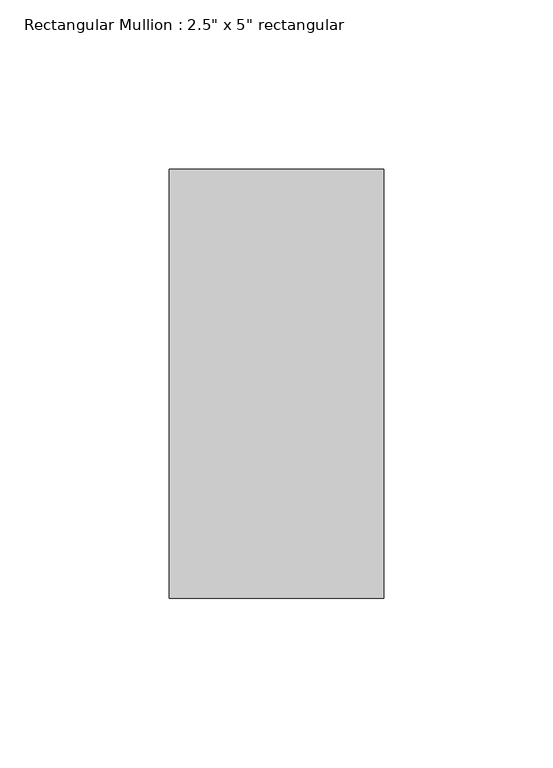
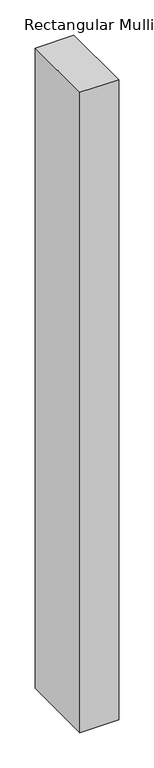
"""IFC4 building model written with IfcOpenShell, lengths in millimetres: member geometry."""

from ifc_helpers import new_model, si_unit, frame, origin, place, context, project, spatial, polyline, outline, extrude, source, transform, mapped, element, save


def member_d6aa3d2f(model_context):
    return source(origin(), model_context, "Body", "SweptSolid", [
        extrude(outline(polyline([(31.75, 63.5), (31.75, -63.5), (-31.75, -63.5), (-31.75, 63.5), (31.75, 63.5)])), frame((0.0, 0.0, -1110.6251745), z_axis=(0.0, 0.0, 1.0), x_axis=(1.0, 0.0, 0.0)), (0.0, 0.0, 1.0), 1110.6251745),
    ])


if __name__ == "__main__":
    model = new_model("IFC4")
    model_context = context("Model", 3, world=origin())
    ifc_project = project(units=[si_unit("LENGTHUNIT", "METRE", prefix="MILLI")], contexts=[model_context])
    site = spatial("IfcSite", under=ifc_project)
    building = spatial("IfcBuilding", under=site)
    placement = place(None, origin())
    member_shape = member_d6aa3d2f(model_context)
    element("IfcMember", 1, ObjectType="Rectangular Mullion : 2.5\" x 5\" rectangular", at=placement, inside=building, context=model_context, shape_type="MappedRepresentation", body=[
        mapped(member_shape, transform((0.0, 0.0, 0.0), x_axis=(1.0, 0.0, 0.0), y_axis=(0.0, 1.0, 0.0), z_axis=(0.0, 0.0, 1.0))),
    ])
    save(model, "model.ifc")

# Revit data of these elements
# Type "Rectangular Mullion : 2.5\" x 5\" rectangular"
#   built-in parameter 1007304 = 0.416667 (stored number, unit not read)
#   built-in parameter 1007301 = 0.104167 (stored number, unit not read)
#   built-in parameter 1007300 = 0.104167 (stored number, unit not read)
# Element 1 (IfcMember, "Rectangular Mullion : 2.5\" x 5\" rectangular")
#   Materials on its faces: "Aluminum"
# Materials
#   "Aluminum": class "Metal", colour RGB 247 247 247, transparency 0, Description = "Aluminum 6061", Cost = 0
